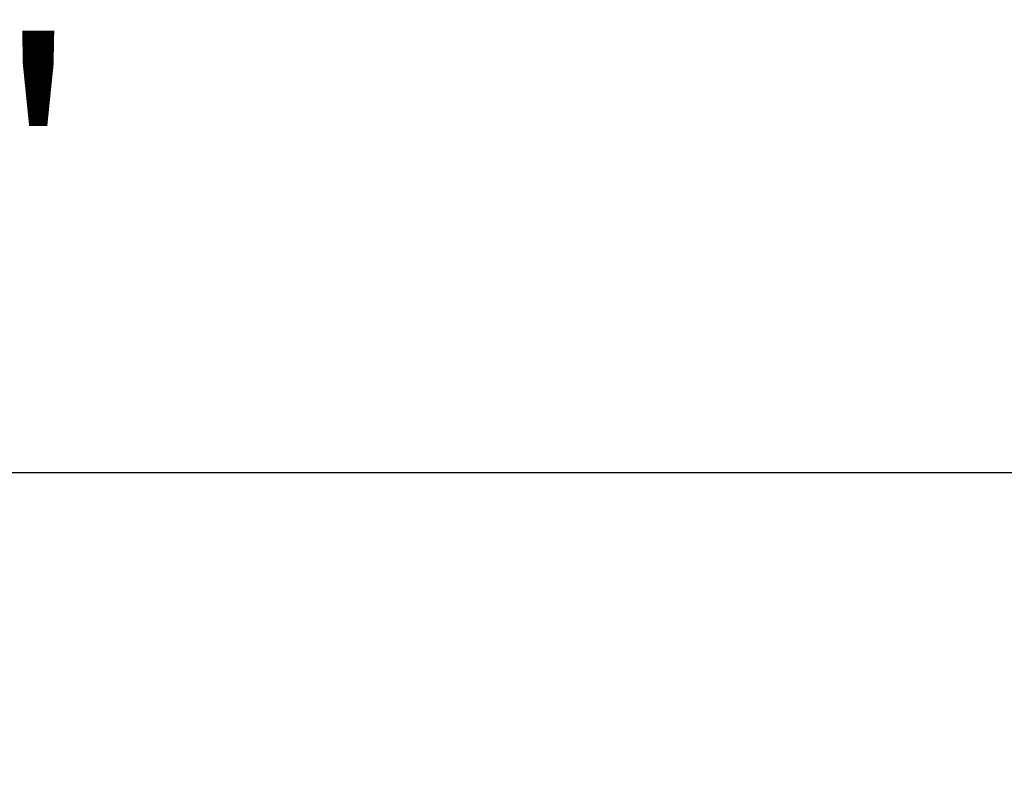
# Model space of a CAD drawing. Units: millimetres. Extents: x 7894 to 8038, y 6851 to 6951.
# Tile 19 of 49: x 7954.632 to 7958.696, y 6903.287 to 6906.405. Entities that reach past the tile are written whole.
import ezdxf

# ---------------------------------------------------------------- set-up
doc = ezdxf.new("R2010")
doc.units = ezdxf.units.MM
doc.layers.add('A-ANNO-DIMS', color=2, linetype='Continuous', lineweight=18)
doc.styles.get("Standard").update_dxf_attribs({"font": 'arial.ttf'})
doc.dimstyles.new('ISO-25', dxfattribs={"dimtxt": 1, "dimasz": 1, "dimexe": 1.25, "dimexo": 0.625, "dimtad": 1, "dimdec": 0, "dimlunit": 4, "dimtxsty": 'Standard', "dimcen": 2.5, "dimclrt": 1, "dimadec": 0, "dimazin": 0, "dimtfac": 1, "dimtdec": 0, "dimtmove": 0, "dimatfit": 3, "dimfxl": 1, "dimarcsym": 0})

# ---------------------------------------------------------------- blocks, each defined once
blk = doc.blocks.new('*D25')
at = {"layer": 'A-ANNO-DIMS', "color": 0, "lineweight": -2, "transparency": 16777216}
for p, q in [((7940.0888, 6905.848), (7940.0888, 6903.2865)), ((7964.3408, 6905.8484), (7964.3408, 6903.2865)), ((7941.0888, 6904.5365), (7963.3408, 6904.5365))]:
    blk.add_line(p, q, dxfattribs=at)
at = {"layer": 'A-ANNO-DIMS', "color": 0, "transparency": 16777216}
for points in [[(7941.0888, 6904.7032), (7941.0888, 6904.3699), (7940.0888, 6904.5365)], [(7963.3408, 6904.7032), (7963.3408, 6904.3699), (7964.3408, 6904.5365)]]:
    blk.add_solid(points, dxfattribs=at)
at = {"layer": 'Defpoints', "color": 0, "transparency": 16777216}
for p in [(7940.0888, 6906.473), (7964.3408, 6906.4734), (7964.3408, 6904.5365)]:
    blk.add_point(p, dxfattribs=at)
at = {"layer": 'A-ANNO-DIMS', "color": 1, "transparency": 16777216, "insert": (7952.2148, 6905.6786), "char_height": 1, "attachment_point": 5}
blk.add_mtext('2\'-0 1/2"', dxfattribs=at)

msp = doc.modelspace()

# ---------------------------------------------------------------- dimensions: what is measured, and where the dimension line sits
at = {"layer": 'A-ANNO-DIMS'}
dim = msp.add_linear_dim(base=(7964.3408, 6904.5365), p1=(7940.0888, 6906.473), p2=(7964.3408, 6906.4734), dimstyle='ISO-25', override={"dimdec": 1, "dimlfac": 1, "dimrnd": 0, "dimzin": 1, "dimdsep": 46, "dimlunit": 4, "dimfrac": 2}, dxfattribs=at)
dim.commit()
dim.dimension.update_dxf_attribs({"geometry": '*D25', "text_midpoint": (7952.2148, 6905.6786)})

doc.saveas('drawing.dxf')
